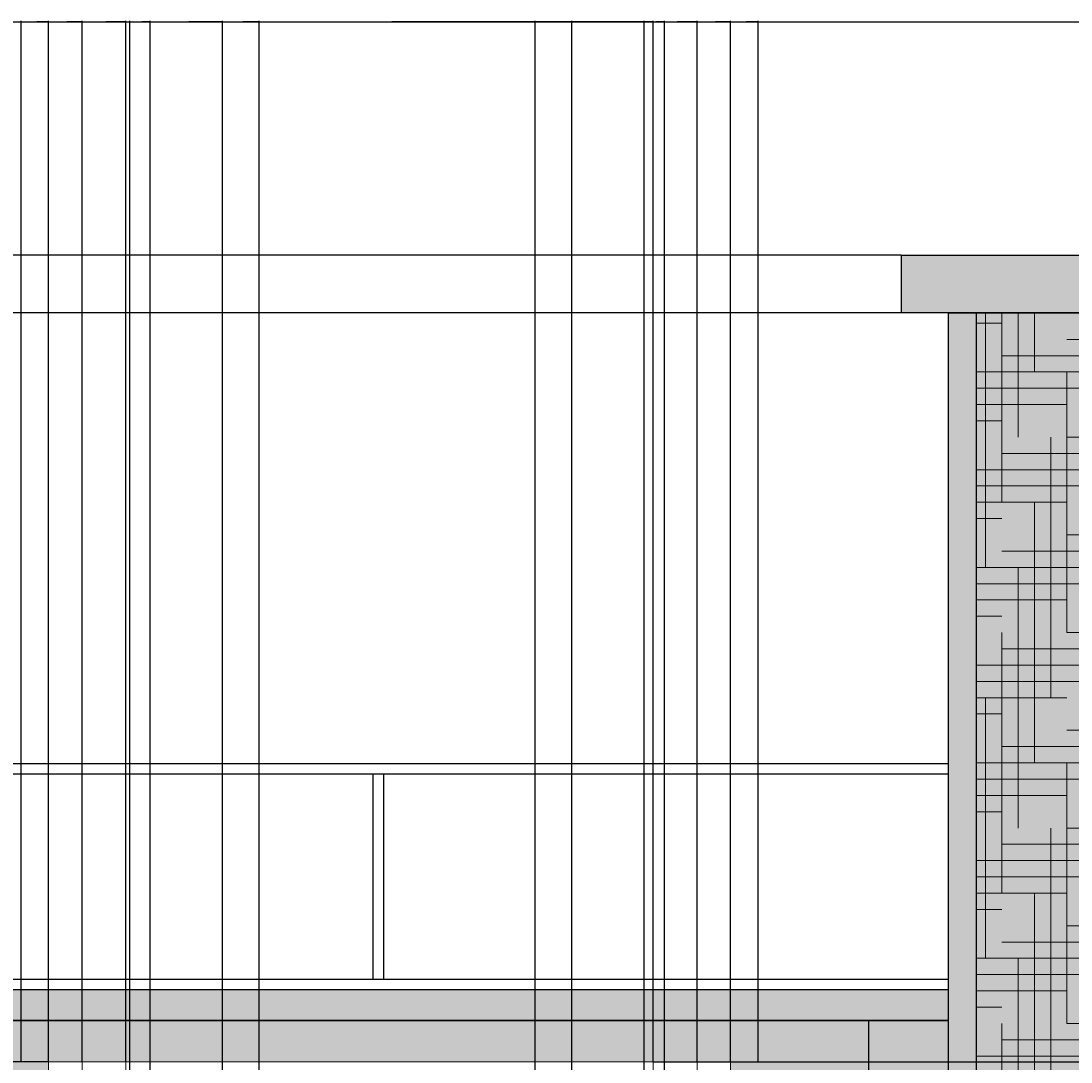
# Model space of a CAD drawing. Units: inches. Extents: x 3024 to 4744, y 1110 to 2100.
# Tile 25 of 29: x 3149 to 3354, y 1897 to 2100. Entities that reach past the tile are written whole.
import ezdxf

# ---------------------------------------------------------------- set-up
doc = ezdxf.new("R2010")
doc.units = ezdxf.units.IN
for name, color, linetype, lineweight in [('A-ANNO-DIMS', 2, 'Continuous', 18), ('A-ELEV', 7, 'Continuous', 25), ('A-ELEV-PATT', 252, 'Continuous', 13), ('A-GLAZ', 4, 'Continuous', 18)]:
    doc.layers.add(name, color=color, linetype=linetype, lineweight=lineweight)
doc.styles.get("Standard").update_dxf_attribs({"font": 'arial.ttf'})
doc.dimstyles.get("Standard").update_dxf_attribs({"dimtxt": 0.18, "dimasz": 0.18, "dimexe": 0.18, "dimexo": 0.0625, "dimgap": 0.09, "dimtad": 0, "dimtih": 1, "dimtoh": 1, "dimdec": 1, "dimzin": 0, "dimdsep": 46, "dimlunit": 3, "dimtxsty": 'Standard', "dimcen": 0.09, "dimadec": 0, "dimazin": 0, "dimtfac": 1, "dimtdec": 1, "dimtofl": 0, "dimtmove": 0, "dimatfit": 3, "dimfxl": 1, "dimtolj": 1, "dimtzin": 0, "dimarcsym": 0})

# ---------------------------------------------------------------- blocks, each defined once
blk = doc.blocks.new('WIN-BALCONY-A')
for p, q in [((3169.4, 1897.49), (3148.97, 1897.49)), ((3169.4, 1897.49), (3148.97, 1897.49)), ((3169.4, 1897.49), (3292.61, 1897.49)), ((3169.4, 1897.49), (3292.61, 1897.49)), ((3169.4, 1795.04), (3148.97, 1795.04)), ((3169.4, 1795.04), (3148.97, 1795.04)), ((3169.4, 1795.04), (3292.61, 1795.04)), ((3169.4, 1795.04), (3292.61, 1795.04))]:
    blk.add_line(p, q)
for points in [[(3148.97, 1897.49), (3148.97, 1905.61), (3292.61, 1905.61), (3292.61, 1897.49)], [(3148.97, 1897.49), (3148.97, 1905.61), (3292.61, 1905.61), (3292.61, 1897.49)], [(3292.61, 1795.04), (3292.61, 1785.61), (3148.97, 1785.61), (3148.97, 1795.04)], [(3292.61, 1795.04), (3292.61, 1785.61), (3148.97, 1785.61), (3148.97, 1795.04)]]:
    blk.add_lwpolyline(points)
for points in [[(3154.33, 1806.87), (3160.86, 1806.87), (3160.86, 1897.49), (3154.33, 1897.49)], [(3154.33, 1806.87), (3160.86, 1806.87), (3160.86, 1897.49), (3154.33, 1897.49)], [(3272.18, 1795.04), (3169.4, 1795.04), (3169.4, 1897.49), (3272.18, 1897.49)], [(3272.18, 1795.04), (3169.4, 1795.04), (3169.4, 1897.49), (3272.18, 1897.49)], [(3287.25, 1806.87), (3280.72, 1806.87), (3280.72, 1897.49), (3287.25, 1897.49)], [(3287.25, 1806.87), (3280.72, 1806.87), (3280.72, 1897.49), (3287.25, 1897.49)], [(3268.18, 1799.04), (3173.4, 1799.04), (3173.4, 1893.49), (3268.18, 1893.49)], [(3268.18, 1799.04), (3173.4, 1799.04), (3173.4, 1893.49), (3268.18, 1893.49)], [(3220.05, 1893.49), (3221.52, 1893.49), (3221.52, 1799.04), (3220.05, 1799.04)], [(3220.05, 1893.49), (3221.52, 1893.49), (3221.52, 1799.04), (3220.05, 1799.04)], [(3163.53, 1795.04), (3151.66, 1795.04), (3151.66, 1806.87), (3163.53, 1806.87)], [(3163.53, 1795.04), (3151.66, 1795.04), (3151.66, 1806.87), (3163.53, 1806.87)], [(3276.51, 1795.04), (3288.38, 1795.04), (3288.38, 1806.87), (3276.51, 1806.87)], [(3276.51, 1795.04), (3288.38, 1795.04), (3288.38, 1806.87), (3276.51, 1806.87)]]:
    blk.add_lwpolyline(points, close=True)
blk = doc.blocks.new('*D7')
at = {"layer": 'A-ANNO-DIMS', "color": 0, "lineweight": -2, "transparency": 16777216}
for p, q in [((3292.67, 1905.61), (3314.33, 1905.61)), ((3314.15, 1905.43), (3314.15, 1845.79)), ((3314.15, 1785.79), (3314.15, 1845.43)), ((3292.67, 1785.61), (3314.33, 1785.61))]:
    blk.add_line(p, q, dxfattribs=at)
at = {"layer": 'A-ANNO-DIMS', "color": 0, "transparency": 16777216}
for points in [[(3314.12, 1905.43), (3314.18, 1905.43), (3314.15, 1905.61)], [(3314.12, 1785.79), (3314.18, 1785.79), (3314.15, 1785.61)]]:
    blk.add_solid(points, dxfattribs=at)
at = {"layer": 'Defpoints', "color": 0, "transparency": 16777216}
for p in [(3292.61, 1905.61), (3314.15, 1905.61), (3292.61, 1785.61)]:
    blk.add_point(p, dxfattribs=at)
at = {"layer": 'A-ANNO-DIMS', "color": 0, "transparency": 16777216, "insert": (3314.15, 1845.61), "char_height": 0.18, "attachment_point": 5}
blk.add_mtext('\\A1;120 TYP.', dxfattribs=at)
blk = doc.blocks.new('*D64')
at = {"layer": 'A-ANNO-DIMS', "color": 0, "lineweight": -2, "transparency": 16777216}
for p, q in [((3069.79, 1241.5), (3069.79, 2100.44)), ((3069.97, 2100.26), (3405.08, 2100.26)), ((3740.97, 2100.26), (3405.87, 2100.26)), ((3741.15, 1241.5), (3741.15, 2100.44))]:
    blk.add_line(p, q, dxfattribs=at)
at = {"layer": 'A-ANNO-DIMS', "color": 0, "transparency": 16777216}
for points in [[(3069.97, 2100.29), (3069.97, 2100.23), (3069.79, 2100.26)], [(3740.97, 2100.29), (3740.97, 2100.23), (3741.15, 2100.26)]]:
    blk.add_solid(points, dxfattribs=at)
at = {"layer": 'Defpoints', "color": 0, "transparency": 16777216}
for p in [(3741.15, 2100.26), (3069.79, 1241.43), (3741.15, 1241.43)]:
    blk.add_point(p, dxfattribs=at)
at = {"layer": 'A-ANNO-DIMS', "color": 0, "transparency": 16777216, "insert": (3405.47, 2100.26), "char_height": 0.18, "attachment_point": 5}
blk.add_mtext('\\A1;671.4', dxfattribs=at)
blk = doc.blocks.new('*D73')
at = {"layer": 'A-ANNO-DIMS', "color": 0, "lineweight": -2, "transparency": 16777216}
for p, q in [((3329.64, 2043.53), (3024.11, 2043.53)), ((3024.29, 2043.35), (3024.29, 1999.76)), ((3024.29, 1955.8), (3024.29, 1999.39)), ((3105.41, 1955.62), (3024.11, 1955.62))]:
    blk.add_line(p, q, dxfattribs=at)
at = {"layer": 'A-ANNO-DIMS', "color": 0, "transparency": 16777216}
for points in [[(3024.26, 2043.35), (3024.32, 2043.35), (3024.29, 2043.53)], [(3024.26, 1955.8), (3024.32, 1955.8), (3024.29, 1955.62)]]:
    blk.add_solid(points, dxfattribs=at)
at = {"layer": 'Defpoints', "color": 0, "transparency": 16777216}
for p in [(3024.29, 2043.53), (3329.7, 2043.53), (3105.47, 1955.62)]:
    blk.add_point(p, dxfattribs=at)
at = {"layer": 'A-ANNO-DIMS', "color": 0, "transparency": 16777216, "insert": (3024.29, 1999.57), "char_height": 0.18, "attachment_point": 5}
blk.add_mtext('\\A1;87.91', dxfattribs=at)
blk = doc.blocks.new('*D74')
at = {"layer": 'A-ANNO-DIMS', "color": 0, "lineweight": -2, "transparency": 16777216}
for p, q in [((3320.5, 2054.76), (3024.11, 2054.76)), ((3024.29, 2054.58), (3024.29, 2049.33)), ((3024.29, 2043.71), (3024.29, 2048.96)), ((3320.5, 2043.53), (3024.11, 2043.53))]:
    blk.add_line(p, q, dxfattribs=at)
at = {"layer": 'A-ANNO-DIMS', "color": 0, "transparency": 16777216}
for points in [[(3024.26, 2054.58), (3024.32, 2054.58), (3024.29, 2054.76)], [(3024.26, 2043.71), (3024.32, 2043.71), (3024.29, 2043.53)]]:
    blk.add_solid(points, dxfattribs=at)
at = {"layer": 'Defpoints', "color": 0, "transparency": 16777216}
for p in [(3024.29, 2054.76), (3320.57, 2054.76), (3320.57, 2043.53)]:
    blk.add_point(p, dxfattribs=at)
at = {"layer": 'A-ANNO-DIMS', "color": 0, "transparency": 16777216, "insert": (3024.29, 2049.14), "char_height": 0.18, "attachment_point": 5}
blk.add_mtext('\\A1;11.23', dxfattribs=at)
blk = doc.blocks.new('*D82')
at = {"layer": 'A-ANNO-DIMS', "color": 0, "lineweight": -2, "transparency": 16777216}
for p, q in [((3148.97, 1897.55), (3148.97, 2100.44)), ((3149.15, 2100.26), (3151.26, 2100.26)), ((3154.15, 2100.26), (3152.04, 2100.26)), ((3154.33, 1897.55), (3154.33, 2100.44))]:
    blk.add_line(p, q, dxfattribs=at)
at = {"layer": 'A-ANNO-DIMS', "color": 0, "transparency": 16777216}
for points in [[(3149.15, 2100.29), (3149.15, 2100.23), (3148.97, 2100.26)], [(3154.15, 2100.29), (3154.15, 2100.23), (3154.33, 2100.26)]]:
    blk.add_solid(points, dxfattribs=at)
at = {"layer": 'Defpoints', "color": 0, "transparency": 16777216}
for p in [(3154.33, 2100.26), (3148.97, 1897.49), (3154.33, 1897.49)]:
    blk.add_point(p, dxfattribs=at)
at = {"layer": 'A-ANNO-DIMS', "color": 0, "transparency": 16777216, "insert": (3151.65, 2100.26), "char_height": 0.18, "attachment_point": 5}
blk.add_mtext('\\A1;5.359', dxfattribs=at)
blk = doc.blocks.new('*D83')
at = {"layer": 'A-ANNO-DIMS', "color": 0, "lineweight": -2, "transparency": 16777216}
for p, q in [((3154.33, 1897.55), (3154.33, 2100.44)), ((3154.51, 2100.26), (3157.27, 2100.26)), ((3160.68, 2100.26), (3157.92, 2100.26)), ((3160.86, 1897.55), (3160.86, 2100.44))]:
    blk.add_line(p, q, dxfattribs=at)
at = {"layer": 'A-ANNO-DIMS', "color": 0, "transparency": 16777216}
for points in [[(3154.51, 2100.29), (3154.51, 2100.23), (3154.33, 2100.26)], [(3160.68, 2100.29), (3160.68, 2100.23), (3160.86, 2100.26)]]:
    blk.add_solid(points, dxfattribs=at)
at = {"layer": 'Defpoints', "color": 0, "transparency": 16777216}
for p in [(3160.86, 2100.26), (3154.33, 1897.49), (3160.86, 1897.49)]:
    blk.add_point(p, dxfattribs=at)
at = {"layer": 'A-ANNO-DIMS', "color": 0, "transparency": 16777216, "insert": (3157.59, 2100.26), "char_height": 0.18, "attachment_point": 5}
blk.add_mtext('\\A1;6.53', dxfattribs=at)
blk = doc.blocks.new('*D84')
at = {"layer": 'A-ANNO-DIMS', "color": 0, "lineweight": -2, "transparency": 16777216}
for p, q in [((3160.86, 1897.55), (3160.86, 2100.44)), ((3161.04, 2100.26), (3164.73, 2100.26)), ((3169.22, 2100.26), (3165.52, 2100.26)), ((3169.4, 1897.55), (3169.4, 2100.44))]:
    blk.add_line(p, q, dxfattribs=at)
at = {"layer": 'A-ANNO-DIMS', "color": 0, "transparency": 16777216}
for points in [[(3161.04, 2100.29), (3161.04, 2100.23), (3160.86, 2100.26)], [(3169.22, 2100.29), (3169.22, 2100.23), (3169.4, 2100.26)]]:
    blk.add_solid(points, dxfattribs=at)
at = {"layer": 'Defpoints', "color": 0, "transparency": 16777216}
for p in [(3169.4, 2100.26), (3160.86, 1897.49), (3169.4, 1897.49)]:
    blk.add_point(p, dxfattribs=at)
at = {"layer": 'A-ANNO-DIMS', "color": 0, "transparency": 16777216, "insert": (3165.13, 2100.26), "char_height": 0.18, "attachment_point": 5}
blk.add_mtext('\\A1;8.538', dxfattribs=at)
blk = doc.blocks.new('*D85')
at = {"layer": 'A-ANNO-DIMS', "color": 0, "lineweight": -2, "transparency": 16777216}
for p, q in [((3169.4, 1897.55), (3169.4, 2100.44)), ((3169.58, 2100.26), (3220.33, 2100.26)), ((3272, 2100.26), (3221.24, 2100.26)), ((3272.18, 1897.55), (3272.18, 2100.44))]:
    blk.add_line(p, q, dxfattribs=at)
at = {"layer": 'A-ANNO-DIMS', "color": 0, "transparency": 16777216}
for points in [[(3169.58, 2100.29), (3169.58, 2100.23), (3169.4, 2100.26)], [(3272, 2100.29), (3272, 2100.23), (3272.18, 2100.26)]]:
    blk.add_solid(points, dxfattribs=at)
at = {"layer": 'Defpoints', "color": 0, "transparency": 16777216}
for p in [(3272.18, 2100.26), (3169.4, 1897.49), (3272.18, 1897.49)]:
    blk.add_point(p, dxfattribs=at)
at = {"layer": 'A-ANNO-DIMS', "color": 0, "transparency": 16777216, "insert": (3220.79, 2100.26), "char_height": 0.18, "attachment_point": 5}
blk.add_mtext('\\A1;102.78', dxfattribs=at)
blk = doc.blocks.new('*D86')
at = {"layer": 'A-ANNO-DIMS', "color": 0, "lineweight": -2, "transparency": 16777216}
for p, q in [((3272.18, 1897.55), (3272.18, 2100.44)), ((3272.36, 2100.26), (3276.05, 2100.26)), ((3280.54, 2100.26), (3276.84, 2100.26)), ((3280.72, 1897.55), (3280.72, 2100.44))]:
    blk.add_line(p, q, dxfattribs=at)
at = {"layer": 'A-ANNO-DIMS', "color": 0, "transparency": 16777216}
for points in [[(3272.36, 2100.29), (3272.36, 2100.23), (3272.18, 2100.26)], [(3280.54, 2100.29), (3280.54, 2100.23), (3280.72, 2100.26)]]:
    blk.add_solid(points, dxfattribs=at)
at = {"layer": 'Defpoints', "color": 0, "transparency": 16777216}
for p in [(3280.72, 2100.26), (3272.18, 1897.49), (3280.72, 1897.49)]:
    blk.add_point(p, dxfattribs=at)
at = {"layer": 'A-ANNO-DIMS', "color": 0, "transparency": 16777216, "insert": (3276.45, 2100.26), "char_height": 0.18, "attachment_point": 5}
blk.add_mtext('\\A1;8.538', dxfattribs=at)
blk = doc.blocks.new('*D87')
at = {"layer": 'A-ANNO-DIMS', "color": 0, "lineweight": -2, "transparency": 16777216}
for p, q in [((3280.72, 1897.55), (3280.72, 2100.44)), ((3280.9, 2100.26), (3283.66, 2100.26)), ((3287.07, 2100.26), (3284.31, 2100.26)), ((3287.25, 1897.55), (3287.25, 2100.44))]:
    blk.add_line(p, q, dxfattribs=at)
at = {"layer": 'A-ANNO-DIMS', "color": 0, "transparency": 16777216}
for points in [[(3280.9, 2100.29), (3280.9, 2100.23), (3280.72, 2100.26)], [(3287.07, 2100.29), (3287.07, 2100.23), (3287.25, 2100.26)]]:
    blk.add_solid(points, dxfattribs=at)
at = {"layer": 'Defpoints', "color": 0, "transparency": 16777216}
for p in [(3287.25, 2100.26), (3280.72, 1897.49), (3287.25, 1897.49)]:
    blk.add_point(p, dxfattribs=at)
at = {"layer": 'A-ANNO-DIMS', "color": 0, "transparency": 16777216, "insert": (3283.98, 2100.26), "char_height": 0.18, "attachment_point": 5}
blk.add_mtext('\\A1;6.53', dxfattribs=at)
blk = doc.blocks.new('*D88')
at = {"layer": 'A-ANNO-DIMS', "color": 0, "lineweight": -2, "transparency": 16777216}
for p, q in [((3287.25, 1897.55), (3287.25, 2100.44)), ((3287.43, 2100.26), (3289.53, 2100.26)), ((3292.43, 2100.26), (3290.32, 2100.26)), ((3292.61, 1897.55), (3292.61, 2100.44))]:
    blk.add_line(p, q, dxfattribs=at)
at = {"layer": 'A-ANNO-DIMS', "color": 0, "transparency": 16777216}
for points in [[(3287.43, 2100.29), (3287.43, 2100.23), (3287.25, 2100.26)], [(3292.43, 2100.29), (3292.43, 2100.23), (3292.61, 2100.26)]]:
    blk.add_solid(points, dxfattribs=at)
at = {"layer": 'Defpoints', "color": 0, "transparency": 16777216}
for p in [(3292.61, 2100.26), (3287.25, 1897.49), (3292.61, 1897.49)]:
    blk.add_point(p, dxfattribs=at)
at = {"layer": 'A-ANNO-DIMS', "color": 0, "transparency": 16777216, "insert": (3289.93, 2100.26), "char_height": 0.18, "attachment_point": 5}
blk.add_mtext('\\A1;5.359', dxfattribs=at)
blk = doc.blocks.new('*D98')
at = {"layer": 'A-ANNO-DIMS', "color": 0, "lineweight": -2, "transparency": 16777216}
for p, q in [((3154.27, 1897.49), (3024.11, 1897.49)), ((3024.29, 1897.31), (3024.29, 1852.36)), ((3024.29, 1807.05), (3024.29, 1852)), ((3154.27, 1806.87), (3024.11, 1806.87))]:
    blk.add_line(p, q, dxfattribs=at)
at = {"layer": 'A-ANNO-DIMS', "color": 0, "transparency": 16777216}
for points in [[(3024.26, 1897.31), (3024.32, 1897.31), (3024.29, 1897.49)], [(3024.26, 1807.05), (3024.32, 1807.05), (3024.29, 1806.87)]]:
    blk.add_solid(points, dxfattribs=at)
at = {"layer": 'Defpoints', "color": 0, "transparency": 16777216}
for p in [(3024.29, 1897.49), (3154.33, 1897.49), (3154.33, 1806.87)]:
    blk.add_point(p, dxfattribs=at)
at = {"layer": 'A-ANNO-DIMS', "color": 0, "transparency": 16777216, "insert": (3024.29, 1852.18), "char_height": 0.18, "attachment_point": 5}
blk.add_mtext('\\A1;90.62', dxfattribs=at)
blk = doc.blocks.new('*D102')
at = {"layer": 'A-ANNO-DIMS', "color": 0, "lineweight": -2, "transparency": 16777216}
for p, q in [((3272.24, 1897.49), (3786.83, 1897.49)), ((3786.65, 1897.31), (3786.65, 1895.67)), ((3786.65, 1893.67), (3786.65, 1895.31)), ((3268.24, 1893.49), (3786.83, 1893.49))]:
    blk.add_line(p, q, dxfattribs=at)
at = {"layer": 'A-ANNO-DIMS', "color": 0, "transparency": 16777216}
for points in [[(3786.62, 1897.31), (3786.68, 1897.31), (3786.65, 1897.49)], [(3786.62, 1893.67), (3786.68, 1893.67), (3786.65, 1893.49)]]:
    blk.add_solid(points, dxfattribs=at)
at = {"layer": 'Defpoints', "color": 0, "transparency": 16777216}
for p in [(3272.18, 1897.49), (3786.65, 1897.49), (3268.18, 1893.49)]:
    blk.add_point(p, dxfattribs=at)
at = {"layer": 'A-ANNO-DIMS', "color": 0, "transparency": 16777216, "insert": (3786.65, 1895.49), "char_height": 0.18, "attachment_point": 5}
blk.add_mtext('\\A1;4.00', dxfattribs=at)
blk = doc.blocks.new('*D106')
at = {"layer": 'A-ANNO-DIMS', "color": 0, "lineweight": -2, "transparency": 16777216}
for p, q in [((3170.16, 1275.67), (3170.16, 2100.44)), ((3170.34, 2100.26), (3171.83, 2100.26)), ((3173.98, 2100.26), (3172.49, 2100.26)), ((3174.16, 1271.67), (3174.16, 2100.44))]:
    blk.add_line(p, q, dxfattribs=at)
at = {"layer": 'A-ANNO-DIMS', "color": 0, "transparency": 16777216}
for points in [[(3170.34, 2100.29), (3170.34, 2100.23), (3170.16, 2100.26)], [(3173.98, 2100.29), (3173.98, 2100.23), (3174.16, 2100.26)]]:
    blk.add_solid(points, dxfattribs=at)
at = {"layer": 'Defpoints', "color": 0, "transparency": 16777216}
for p in [(3174.16, 2100.26), (3170.16, 1275.61), (3174.16, 1271.61)]:
    blk.add_point(p, dxfattribs=at)
at = {"layer": 'A-ANNO-DIMS', "color": 0, "transparency": 16777216, "insert": (3172.16, 2100.26), "char_height": 0.18, "attachment_point": 5}
blk.add_mtext('\\A1;4.00', dxfattribs=at)
blk = doc.blocks.new('*D107')
at = {"layer": 'A-ANNO-DIMS', "color": 0, "lineweight": -2, "transparency": 16777216}
for p, q in [((3174.16, 1271.67), (3174.16, 2100.44)), ((3174.34, 2100.26), (3221.88, 2100.26)), ((3270.21, 2100.26), (3222.67, 2100.26)), ((3270.39, 1271.67), (3270.39, 2100.44))]:
    blk.add_line(p, q, dxfattribs=at)
at = {"layer": 'A-ANNO-DIMS', "color": 0, "transparency": 16777216}
for points in [[(3174.34, 2100.29), (3174.34, 2100.23), (3174.16, 2100.26)], [(3270.21, 2100.29), (3270.21, 2100.23), (3270.39, 2100.26)]]:
    blk.add_solid(points, dxfattribs=at)
at = {"layer": 'Defpoints', "color": 0, "transparency": 16777216}
for p in [(3270.39, 2100.26), (3174.16, 1271.61), (3270.39, 1271.61)]:
    blk.add_point(p, dxfattribs=at)
at = {"layer": 'A-ANNO-DIMS', "color": 0, "transparency": 16777216, "insert": (3222.27, 2100.26), "char_height": 0.18, "attachment_point": 5}
blk.add_mtext('\\A1;96.23', dxfattribs=at)
blk = doc.blocks.new('*D108')
at = {"layer": 'A-ANNO-DIMS', "color": 0, "lineweight": -2, "transparency": 16777216}
for p, q in [((3270.39, 1271.67), (3270.39, 2100.44)), ((3270.57, 2100.26), (3272.06, 2100.26)), ((3274.21, 2100.26), (3272.71, 2100.26)), ((3274.39, 1275.67), (3274.39, 2100.44))]:
    blk.add_line(p, q, dxfattribs=at)
at = {"layer": 'A-ANNO-DIMS', "color": 0, "transparency": 16777216}
for points in [[(3270.57, 2100.29), (3270.57, 2100.23), (3270.39, 2100.26)], [(3274.21, 2100.29), (3274.21, 2100.23), (3274.39, 2100.26)]]:
    blk.add_solid(points, dxfattribs=at)
at = {"layer": 'Defpoints', "color": 0, "transparency": 16777216}
for p in [(3274.39, 2100.26), (3274.39, 1275.61), (3270.39, 1271.61)]:
    blk.add_point(p, dxfattribs=at)
at = {"layer": 'A-ANNO-DIMS', "color": 0, "transparency": 16777216, "insert": (3272.39, 2100.26), "char_height": 0.18, "attachment_point": 5}
blk.add_mtext('\\A1;4.00', dxfattribs=at)
blk = doc.blocks.new('*D124')
at = {"layer": 'A-ANNO-DIMS', "color": 0, "lineweight": -2, "transparency": 16777216}
for p, q in [((3174.16, 1271.67), (3174.16, 2100.44)), ((3174.34, 2100.26), (3180.75, 2100.26)), ((3188.08, 2100.26), (3181.67, 2100.26)), ((3188.26, 1256.29), (3188.26, 2100.44))]:
    blk.add_line(p, q, dxfattribs=at)
at = {"layer": 'A-ANNO-DIMS', "color": 0, "transparency": 16777216}
for points in [[(3174.34, 2100.29), (3174.34, 2100.23), (3174.16, 2100.26)], [(3188.08, 2100.29), (3188.08, 2100.23), (3188.26, 2100.26)]]:
    blk.add_solid(points, dxfattribs=at)
at = {"layer": 'Defpoints', "color": 0, "transparency": 16777216}
for p in [(3188.26, 2100.26), (3174.16, 1271.61), (3188.26, 1256.23)]:
    blk.add_point(p, dxfattribs=at)
at = {"layer": 'A-ANNO-DIMS', "color": 0, "transparency": 16777216, "insert": (3181.21, 2100.26), "char_height": 0.18, "attachment_point": 5}
blk.add_mtext('\\A1;14.098', dxfattribs=at)
blk = doc.blocks.new('*D125')
at = {"layer": 'A-ANNO-DIMS', "color": 0, "lineweight": -2, "transparency": 16777216}
for p, q in [((3188.26, 1256.29), (3188.26, 2100.44)), ((3188.44, 2100.26), (3191.44, 2100.26)), ((3195.23, 2100.26), (3192.22, 2100.26)), ((3195.41, 1256.29), (3195.41, 2100.44))]:
    blk.add_line(p, q, dxfattribs=at)
at = {"layer": 'A-ANNO-DIMS', "color": 0, "transparency": 16777216}
for points in [[(3188.44, 2100.29), (3188.44, 2100.23), (3188.26, 2100.26)], [(3195.23, 2100.29), (3195.23, 2100.23), (3195.41, 2100.26)]]:
    blk.add_solid(points, dxfattribs=at)
at = {"layer": 'Defpoints', "color": 0, "transparency": 16777216}
for p in [(3195.41, 2100.26), (3188.26, 1256.23), (3195.41, 1256.23)]:
    blk.add_point(p, dxfattribs=at)
at = {"layer": 'A-ANNO-DIMS', "color": 0, "transparency": 16777216, "insert": (3191.83, 2100.26), "char_height": 0.18, "attachment_point": 5}
blk.add_mtext('\\A1;7.147', dxfattribs=at)
blk = doc.blocks.new('*D126')
at = {"layer": 'A-ANNO-DIMS', "color": 0, "lineweight": -2, "transparency": 16777216}
for p, q in [((3249.14, 1256.29), (3249.14, 2100.44)), ((3249.32, 2100.26), (3252.32, 2100.26)), ((3256.11, 2100.26), (3253.11, 2100.26)), ((3256.29, 1256.29), (3256.29, 2100.44))]:
    blk.add_line(p, q, dxfattribs=at)
at = {"layer": 'A-ANNO-DIMS', "color": 0, "transparency": 16777216}
for points in [[(3249.32, 2100.29), (3249.32, 2100.23), (3249.14, 2100.26)], [(3256.11, 2100.29), (3256.11, 2100.23), (3256.29, 2100.26)]]:
    blk.add_solid(points, dxfattribs=at)
at = {"layer": 'Defpoints', "color": 0, "transparency": 16777216}
for p in [(3256.29, 2100.26), (3249.14, 1256.23), (3256.29, 1256.23)]:
    blk.add_point(p, dxfattribs=at)
at = {"layer": 'A-ANNO-DIMS', "color": 0, "transparency": 16777216, "insert": (3252.72, 2100.26), "char_height": 0.18, "attachment_point": 5}
blk.add_mtext('\\A1;7.147', dxfattribs=at)

msp = doc.modelspace()

# ---------------------------------------------------------------- hatches: boundary and pattern name
at = {"layer": 'A-ELEV-PATT'}
h = msp.add_hatch(color=256, dxfattribs=at)
h.dxf.hatch_style = 1
h.paths.add_polyline_path([(3491.8271, 2054.7584), (3320.5658, 2054.7584), (3320.5658, 2043.5286), (3491.8271, 2043.5286)])
h.paths.add_polyline_path([(3292.6051, 1905.6112), (3148.9694, 1905.6112), (3148.9694, 1897.4879), (3169.3964, 1897.4879), (3292.6051, 1897.4879)])
h.paths.add_polyline_path([(3292.6051, 1795.0431), (3169.3964, 1795.0431), (3148.9694, 1795.0431), (3148.9694, 1785.6112), (3292.6051, 1785.6112)])
h.paths.add_polyline_path([(3292.6051, 1779.6112), (3148.9694, 1779.6112), (3148.9694, 1771.4879), (3169.3964, 1771.4879), (3292.6051, 1771.4879)])
h.paths.add_polyline_path([(3292.6051, 1669.0431), (3169.3964, 1669.0431), (3148.9694, 1669.0431), (3148.9694, 1659.6112), (3292.6051, 1659.6112)])
h.paths.add_polyline_path([(3292.6051, 1653.6112), (3148.9694, 1653.6112), (3148.9694, 1645.4879), (3169.3964, 1645.4879), (3292.6051, 1645.4879)])
h.paths.add_polyline_path([(3292.6051, 1543.0431), (3169.3964, 1543.0431), (3148.9694, 1543.0431), (3148.9694, 1533.6112), (3292.6051, 1533.6112)])
h.paths.add_polyline_path([(3292.6051, 1527.6112), (3148.9694, 1527.6112), (3148.9694, 1519.4879), (3169.3964, 1519.4879), (3292.6051, 1519.4879)])
h.paths.add_polyline_path([(3292.6051, 1401.6112), (3148.9694, 1401.6112), (3148.9694, 1393.4879), (3169.3964, 1393.4879), (3292.6051, 1393.4879)])
h.paths.add_polyline_path([(3292.6051, 1417.0431), (3169.3964, 1417.0431), (3148.9694, 1417.0431), (3148.9694, 1407.6112), (3292.6051, 1407.6112)])
h.paths.add_polyline_path([(3292.6051, 1291.0431), (3169.3964, 1291.0431), (3148.9694, 1291.0431), (3148.9694, 1281.6112), (3292.6051, 1281.6112)])
h.paths.add_polyline_path([(3654.037, 1165.0431), (3530.8283, 1165.0431), (3510.4013, 1165.0431), (3510.4013, 1155.6112), (3654.037, 1155.6112)])
h.paths.add_polyline_path([(3654.037, 1275.6112), (3510.4013, 1275.6112), (3510.4013, 1267.4879), (3530.8283, 1267.4879), (3654.037, 1267.4879)])
h.paths.add_polyline_path([(3654.037, 1291.0431), (3530.8283, 1291.0431), (3510.4013, 1291.0431), (3510.4013, 1281.6112), (3654.037, 1281.6112)])
h.paths.add_polyline_path([(3654.037, 1417.0431), (3530.8283, 1417.0431), (3510.4013, 1417.0431), (3510.4013, 1407.6112), (3654.037, 1407.6112)])
h.paths.add_polyline_path([(3654.037, 1401.6112), (3510.4013, 1401.6112), (3510.4013, 1393.4879), (3530.8283, 1393.4879), (3654.037, 1393.4879)])
h.paths.add_polyline_path([(3654.037, 1543.0431), (3530.8283, 1543.0431), (3510.4013, 1543.0431), (3510.4013, 1533.6112), (3654.037, 1533.6112)])
h.paths.add_polyline_path([(3654.037, 1527.6112), (3510.4013, 1527.6112), (3510.4013, 1519.4879), (3530.8283, 1519.4879), (3654.037, 1519.4879)])
h.paths.add_polyline_path([(3654.037, 1653.6112), (3510.4013, 1653.6112), (3510.4013, 1645.4879), (3530.8283, 1645.4879), (3654.037, 1645.4879)])
h.paths.add_polyline_path([(3654.037, 1669.0431), (3530.8283, 1669.0431), (3510.4013, 1669.0431), (3510.4013, 1659.6112), (3654.037, 1659.6112)])
h.paths.add_polyline_path([(3654.037, 1779.6112), (3510.4013, 1779.6112), (3510.4013, 1771.4879), (3530.8283, 1771.4879), (3654.037, 1771.4879)])
h.paths.add_polyline_path([(3654.037, 1795.0431), (3530.8283, 1795.0431), (3510.4013, 1795.0431), (3510.4013, 1785.6112), (3654.037, 1785.6112)])
h.paths.add_polyline_path([(3654.037, 1905.6112), (3510.4013, 1905.6112), (3510.4013, 1897.4879), (3530.8283, 1897.4879), (3654.037, 1897.4879)])
h = msp.add_hatch(color=256, dxfattribs=at)
h.dxf.hatch_style = 1
h.paths.add_polyline_path([(3335.1044, 2043.5286), (3329.7033, 2043.5286), (3329.7033, 1155.6112), (3335.1044, 1155.6112)])
h.paths.add_polyline_path([(3481.2411, 2043.5286), (3335.1044, 2043.5286), (3335.1044, 1155.6112), (3481.2411, 1155.6112)])
h.paths.add_polyline_path([(3449.7202, 1329.5246), (3361.2242, 1329.5246), (3361.2242, 1436.6064), (3449.7202, 1436.6064)], flags=16)
h.paths.add_polyline_path([(3445.7202, 1333.5246), (3365.2242, 1333.5246), (3365.2242, 1432.6064), (3445.7202, 1432.6064)], flags=0)
h.paths.add_polyline_path([(3449.7202, 1455.5246), (3361.2242, 1455.5246), (3361.2242, 1562.6064), (3449.7202, 1562.6064)], flags=16)
h.paths.add_polyline_path([(3445.7202, 1459.5246), (3365.2242, 1459.5246), (3365.2242, 1558.6064), (3445.7202, 1558.6064)], flags=0)
h.paths.add_polyline_path([(3449.7202, 1581.5246), (3361.2242, 1581.5246), (3361.2242, 1688.6064), (3449.7202, 1688.6064)], flags=16)
h.paths.add_polyline_path([(3445.7202, 1585.5246), (3365.2242, 1585.5246), (3365.2242, 1684.6064), (3445.7202, 1684.6064)], flags=0)
h.paths.add_polyline_path([(3449.7202, 1707.5246), (3361.2242, 1707.5246), (3361.2242, 1814.6064), (3449.7202, 1814.6064)], flags=16)
h.paths.add_polyline_path([(3445.7202, 1711.5246), (3365.2242, 1711.5246), (3365.2242, 1810.6064), (3445.7202, 1810.6064)], flags=0)
h.paths.add_polyline_path([(3449.7202, 1833.5246), (3361.2242, 1833.5246), (3361.2242, 1940.6064), (3449.7202, 1940.6064)], flags=16)
h.paths.add_polyline_path([(3445.7202, 1837.5246), (3365.2242, 1837.5246), (3365.2242, 1936.6064), (3445.7202, 1936.6064)], flags=0)
h = msp.add_hatch(color=256, dxfattribs=at)
h.dxf.hatch_style = 1
h.paths.add_polyline_path([(3475.84, 2043.5286), (3335.1044, 2043.5286), (3335.1044, 1155.6112), (3475.84, 1155.6112)])
h.paths.add_polyline_path([(3449.7202, 1940.6064), (3449.7202, 1833.5246), (3361.2242, 1833.5246), (3361.2242, 1940.6064)], flags=16)
h.paths.add_polyline_path([(3445.7202, 1936.6064), (3445.7202, 1837.5246), (3365.2242, 1837.5246), (3365.2242, 1936.6064)], flags=0)
h.paths.add_polyline_path([(3449.7202, 1814.6064), (3449.7202, 1707.5246), (3361.2242, 1707.5246), (3361.2242, 1814.6064)], flags=16)
h.paths.add_polyline_path([(3445.7202, 1810.6064), (3445.7202, 1711.5246), (3365.2242, 1711.5246), (3365.2242, 1810.6064)], flags=0)
h.paths.add_polyline_path([(3449.7202, 1688.6064), (3449.7202, 1581.5246), (3361.2242, 1581.5246), (3361.2242, 1688.6064)], flags=16)
h.paths.add_polyline_path([(3445.7202, 1684.6064), (3445.7202, 1585.5246), (3365.2242, 1585.5246), (3365.2242, 1684.6064)], flags=0)
h.paths.add_polyline_path([(3449.7202, 1562.6064), (3449.7202, 1455.5246), (3361.2242, 1455.5246), (3361.2242, 1562.6064)], flags=16)
h.paths.add_polyline_path([(3445.7202, 1558.6064), (3445.7202, 1459.5246), (3365.2242, 1459.5246), (3365.2242, 1558.6064)], flags=0)
h.paths.add_polyline_path([(3449.7202, 1436.6064), (3449.7202, 1329.5246), (3361.2242, 1329.5246), (3361.2242, 1436.6064)], flags=16)
h.paths.add_polyline_path([(3445.7202, 1432.6064), (3445.7202, 1333.5246), (3365.2242, 1333.5246), (3365.2242, 1432.6064)], flags=0)
h = msp.add_hatch(dxfattribs=at)
h.set_pattern_fill('HOUND', color=256, scale=2)
h.paths.add_polyline_path([(3475.84, 2043.5286), (3335.1044, 2043.5286), (3335.1044, 1155.6112), (3475.84, 1155.6112)])
h.paths.add_polyline_path([(3449.7202, 1940.6064), (3449.7202, 1833.5246), (3361.2242, 1833.5246), (3361.2242, 1940.6064)], flags=16)
h.paths.add_polyline_path([(3445.7202, 1936.6064), (3445.7202, 1837.5246), (3365.2242, 1837.5246), (3365.2242, 1936.6064)], flags=0)
h.paths.add_polyline_path([(3449.7202, 1814.6064), (3449.7202, 1707.5246), (3361.2242, 1707.5246), (3361.2242, 1814.6064)], flags=16)
h.paths.add_polyline_path([(3445.7202, 1810.6064), (3445.7202, 1711.5246), (3365.2242, 1711.5246), (3365.2242, 1810.6064)], flags=0)
h.paths.add_polyline_path([(3449.7202, 1688.6064), (3449.7202, 1581.5246), (3361.2242, 1581.5246), (3361.2242, 1688.6064)], flags=16)
h.paths.add_polyline_path([(3445.7202, 1684.6064), (3445.7202, 1585.5246), (3365.2242, 1585.5246), (3365.2242, 1684.6064)], flags=0)
h.paths.add_polyline_path([(3449.7202, 1562.6064), (3449.7202, 1455.5246), (3361.2242, 1455.5246), (3361.2242, 1562.6064)], flags=16)
h.paths.add_polyline_path([(3445.7202, 1558.6064), (3445.7202, 1459.5246), (3365.2242, 1459.5246), (3365.2242, 1558.6064)], flags=0)
h.paths.add_polyline_path([(3449.7202, 1436.6064), (3449.7202, 1329.5246), (3361.2242, 1329.5246), (3361.2242, 1436.6064)], flags=16)
h.paths.add_polyline_path([(3445.7202, 1432.6064), (3445.7202, 1333.5246), (3365.2242, 1333.5246), (3365.2242, 1432.6064)], flags=0)
h = msp.add_hatch(color=256, dxfattribs=at)
h.dxf.hatch_style = 1
h.paths.add_polyline_path([(3221.5241, 2019.4879), (3220.0505, 2019.4879), (3220.0505, 1925.0431), (3221.5241, 1925.0431)], flags=0)
h.paths.add_polyline_path([(3221.5241, 2019.4879), (3221.5241, 1925.0431), (3220.0505, 1925.0431), (3220.0505, 2019.4879)], flags=0)
h.paths.add_polyline_path([(3221.5241, 1893.4879), (3220.0505, 1893.4879), (3220.0505, 1799.0431), (3221.5241, 1799.0431)])
h = msp.add_hatch(color=256, dxfattribs=at)
h.dxf.hatch_style = 1
h.paths.add_polyline_path([(3329.7033, 1407.6112), (3105.4722, 1407.6112), (3105.4722, 1401.6112), (3329.7033, 1401.6112)])
h.paths.add_polyline_path([(3329.7033, 1281.6112), (3105.4722, 1281.6112), (3105.4722, 1275.6112), (3112.3838, 1275.6112), (3329.7033, 1275.6112)])
h.paths.add_polyline_path([(3329.7033, 1533.6112), (3105.4722, 1533.6112), (3105.4722, 1527.6112), (3329.7033, 1527.6112)])
h.paths.add_polyline_path([(3329.7033, 1659.6112), (3105.4722, 1659.6112), (3105.4722, 1653.6112), (3329.7033, 1653.6112)])
h.paths.add_polyline_path([(3329.7033, 1785.6112), (3105.4722, 1785.6112), (3105.4722, 1779.6112), (3329.7033, 1779.6112)])
h.paths.add_polyline_path([(3329.7033, 1911.6112), (3105.4722, 1911.6112), (3095.7158, 1911.6112), (3095.7158, 1905.6112), (3329.7033, 1905.6112)])
h.paths.add_polyline_path([(3715.2286, 1911.6112), (3705.4722, 1911.6112), (3705.4722, 1905.6112), (3715.2286, 1905.6112)])
h.paths.add_polyline_path([(3688.5588, 1911.6112), (3481.2411, 1911.6112), (3481.2411, 1905.6112), (3688.5588, 1905.6112)])
h = msp.add_hatch(color=256, dxfattribs=at)
h.dxf.hatch_style = 1
h.paths.add_polyline_path([(3154.3287, 1897.4879), (3148.9694, 1897.4879), (3148.9694, 1905.6112), (3105.4722, 1905.6112), (3105.4722, 1785.6112), (3148.9694, 1785.6112), (3148.9694, 1795.0431), (3151.6604, 1795.0431), (3151.6604, 1806.8674), (3154.3287, 1806.8674)])
h.paths.add_polyline_path([(3329.7033, 1905.6112), (3292.6051, 1905.6112), (3292.6051, 1897.4879), (3287.2458, 1897.4879), (3287.2458, 1806.8674), (3288.3759, 1806.8674), (3288.3759, 1795.0431), (3292.6051, 1795.0431), (3292.6051, 1785.6112), (3329.7033, 1785.6112)])
h.paths.add_polyline_path([(3154.3287, 1771.4879), (3148.9694, 1771.4879), (3148.9694, 1779.6112), (3105.4722, 1779.6112), (3105.4722, 1659.6112), (3148.9694, 1659.6112), (3148.9694, 1669.0431), (3151.6604, 1669.0431), (3151.6604, 1680.8674), (3154.3287, 1680.8674)])
h.paths.add_polyline_path([(3329.7033, 1779.6112), (3292.6051, 1779.6112), (3292.6051, 1771.4879), (3287.2458, 1771.4879), (3287.2458, 1680.8674), (3288.3759, 1680.8674), (3288.3759, 1669.0431), (3292.6051, 1669.0431), (3292.6051, 1659.6112), (3329.7033, 1659.6112)])
h.paths.add_polyline_path([(3154.3287, 1645.4879), (3148.9694, 1645.4879), (3148.9694, 1653.6112), (3105.4722, 1653.6112), (3105.4722, 1533.6112), (3148.9694, 1533.6112), (3148.9694, 1543.0431), (3151.6604, 1543.0431), (3151.6604, 1554.8674), (3154.3287, 1554.8674)])
h.paths.add_polyline_path([(3329.7033, 1653.6112), (3292.6051, 1653.6112), (3292.6051, 1645.4879), (3287.2458, 1645.4879), (3287.2458, 1554.8674), (3288.3759, 1554.8674), (3288.3759, 1543.0431), (3292.6051, 1543.0431), (3292.6051, 1533.6112), (3329.7033, 1533.6112)])
h.paths.add_polyline_path([(3329.7033, 1527.6112), (3292.6051, 1527.6112), (3292.6051, 1519.4879), (3287.2458, 1519.4879), (3287.2458, 1428.8674), (3288.3759, 1428.8674), (3288.3759, 1417.0431), (3292.6051, 1417.0431), (3292.6051, 1407.6112), (3329.7033, 1407.6112)])
h.paths.add_polyline_path([(3329.7033, 1401.6112), (3292.6051, 1401.6112), (3292.6051, 1393.4879), (3287.2458, 1393.4879), (3287.2458, 1302.8674), (3288.3759, 1302.8674), (3288.3759, 1291.0431), (3292.6051, 1291.0431), (3292.6051, 1281.6112), (3329.7033, 1281.6112)])
h.paths.add_polyline_path([(3154.3287, 1393.4879), (3148.9694, 1393.4879), (3148.9694, 1401.6112), (3105.4722, 1401.6112), (3105.4722, 1281.6112), (3148.9694, 1281.6112), (3148.9694, 1291.0431), (3151.6604, 1291.0431), (3151.6604, 1302.8674), (3154.3287, 1302.8674)])
h.paths.add_polyline_path([(3154.3287, 1519.4879), (3148.9694, 1519.4879), (3148.9694, 1527.6112), (3105.4722, 1527.6112), (3105.4722, 1407.6112), (3148.9694, 1407.6112), (3148.9694, 1417.0431), (3151.6604, 1417.0431), (3151.6604, 1428.8674), (3154.3287, 1428.8674)])
h.paths.add_polyline_path([(3515.7606, 1897.4879), (3510.4013, 1897.4879), (3510.4013, 1905.6112), (3481.2411, 1905.6112), (3481.2411, 1785.6112), (3510.4013, 1785.6112), (3510.4013, 1795.0431), (3513.0923, 1795.0431), (3513.0923, 1806.8674), (3515.7606, 1806.8674)])
h.paths.add_polyline_path([(3688.5588, 1905.6112), (3654.037, 1905.6112), (3654.037, 1897.4879), (3648.6777, 1897.4879), (3648.6777, 1806.8674), (3649.8078, 1806.8674), (3649.8078, 1795.0431), (3654.037, 1795.0431), (3654.037, 1785.6112), (3688.5588, 1785.6112)])
h.paths.add_polyline_path([(3515.7606, 1771.4879), (3510.4013, 1771.4879), (3510.4013, 1779.6112), (3481.2411, 1779.6112), (3481.2411, 1659.6112), (3510.4013, 1659.6112), (3510.4013, 1669.0431), (3513.0923, 1669.0431), (3513.0923, 1680.8674), (3515.7606, 1680.8674)])
h.paths.add_polyline_path([(3688.5588, 1779.6112), (3654.037, 1779.6112), (3654.037, 1771.4879), (3648.6777, 1771.4879), (3648.6777, 1680.8674), (3649.8078, 1680.8674), (3649.8078, 1669.0431), (3654.037, 1669.0431), (3654.037, 1659.6112), (3688.5588, 1659.6112)])
h.paths.add_polyline_path([(3515.7606, 1645.4879), (3510.4013, 1645.4879), (3510.4013, 1653.6112), (3481.2411, 1653.6112), (3481.2411, 1533.6112), (3510.4013, 1533.6112), (3510.4013, 1543.0431), (3513.0923, 1543.0431), (3513.0923, 1554.8674), (3515.7606, 1554.8674)])
h.paths.add_polyline_path([(3688.5588, 1653.6112), (3654.037, 1653.6112), (3654.037, 1645.4879), (3648.6777, 1645.4879), (3648.6777, 1554.8674), (3649.8078, 1554.8674), (3649.8078, 1543.0431), (3654.037, 1543.0431), (3654.037, 1533.6112), (3688.5588, 1533.6112)])
h.paths.add_polyline_path([(3515.7606, 1519.4879), (3510.4013, 1519.4879), (3510.4013, 1527.6112), (3481.2411, 1527.6112), (3481.2411, 1407.6112), (3510.4013, 1407.6112), (3510.4013, 1417.0431), (3513.0923, 1417.0431), (3513.0923, 1428.8674), (3515.7606, 1428.8674)])
h.paths.add_polyline_path([(3688.5588, 1527.6112), (3654.037, 1527.6112), (3654.037, 1519.4879), (3648.6777, 1519.4879), (3648.6777, 1428.8674), (3649.8078, 1428.8674), (3649.8078, 1417.0431), (3654.037, 1417.0431), (3654.037, 1407.6112), (3688.5588, 1407.6112)])
h.paths.add_polyline_path([(3515.7606, 1393.4879), (3510.4013, 1393.4879), (3510.4013, 1401.6112), (3481.2411, 1401.6112), (3481.2411, 1281.6112), (3510.4013, 1281.6112), (3510.4013, 1291.0431), (3513.0923, 1291.0431), (3513.0923, 1302.8674), (3515.7606, 1302.8674)])
h.paths.add_polyline_path([(3688.5588, 1401.6112), (3654.037, 1401.6112), (3654.037, 1393.4879), (3648.6777, 1393.4879), (3648.6777, 1302.8674), (3649.8078, 1302.8674), (3649.8078, 1291.0431), (3654.037, 1291.0431), (3654.037, 1281.6112), (3688.5588, 1281.6112)])
h.paths.add_polyline_path([(3515.7606, 1267.4879), (3510.4013, 1267.4879), (3510.4013, 1275.6112), (3481.2411, 1275.6112), (3481.2411, 1155.6112), (3510.4013, 1155.6112), (3510.4013, 1165.0431), (3513.0923, 1165.0431), (3513.0923, 1176.8674), (3515.7606, 1176.8674)])
h.paths.add_polyline_path([(3688.5588, 1275.6112), (3654.037, 1275.6112), (3654.037, 1267.4879), (3648.6777, 1267.4879), (3648.6777, 1176.8674), (3649.8078, 1176.8674), (3649.8078, 1165.0431), (3654.037, 1165.0431), (3654.037, 1155.6112), (3688.5588, 1155.6112)])
h.paths.add_polyline_path([(3112.3838, 1275.6112), (3105.4722, 1275.6112), (3105.4722, 1171.0239), (3112.3838, 1171.0239)])

# ---------------------------------------------------------------- linework, layer by layer
at = {"layer": 'A-ELEV'}
for p, q in [((3095.7158, 1911.6112), (3329.7033, 1911.6112)), ((3095.7158, 1911.6112), (3329.7033, 1911.6112)), ((3329.7033, 1905.6112), (3105.4722, 1905.6112)), ((3329.7033, 1905.6112), (3105.4722, 1905.6112))]:
    msp.add_line(p, q, dxfattribs=at)
for points in [[(3491.8271, 2043.5286), (3320.5658, 2043.5286), (3320.5658, 2054.7584), (3491.8271, 2054.7584)], [(3491.8271, 2043.5286), (3320.5658, 2043.5286), (3320.5658, 2054.7584), (3491.8271, 2054.7584)], [(3481.2411, 1155.6112), (3329.7033, 1155.6112), (3329.7033, 2043.5286), (3481.2411, 2043.5286)], [(3329.7033, 2043.5286), (3335.1044, 2043.5286), (3335.1044, 1155.6112), (3329.7033, 1155.6112)], [(3481.2411, 1155.6112), (3329.7033, 1155.6112), (3329.7033, 2043.5286), (3481.2411, 2043.5286)], [(3329.7033, 2043.5286), (3335.1044, 2043.5286), (3335.1044, 1155.6112), (3329.7033, 1155.6112)]]:
    msp.add_lwpolyline(points, close=True, dxfattribs=at)
for points in [[(3329.7033, 1955.6193), (3105.4722, 1955.6193), (3105.4722, 1911.6112), (3329.7033, 1911.6112)], [(3329.7033, 1955.6193), (3105.4722, 1955.6193), (3105.4722, 1911.6112), (3329.7033, 1911.6112)], [(3329.7033, 1953.6193), (3107.4722, 1953.6193), (3107.4722, 1913.6112), (3329.7033, 1913.6112)], [(3329.7033, 1953.6193), (3107.4722, 1953.6193), (3107.4722, 1913.6112), (3329.7033, 1913.6112)], [(3217.5877, 1913.6112), (3217.5877, 1953.6193)], [(3217.5877, 1913.6112), (3217.5877, 1953.6193)], [(3219.5877, 1953.6193), (3219.5877, 1913.6112)], [(3219.5877, 1953.6193), (3219.5877, 1913.6112)], [(3095.7158, 1911.6112), (3095.7158, 1905.6112), (3329.7033, 1905.6112), (3329.7033, 1911.6112)], [(3095.7158, 1911.6112), (3095.7158, 1905.6112), (3329.7033, 1905.6112), (3329.7033, 1911.6112)]]:
    msp.add_lwpolyline(points, dxfattribs=at)

# ---------------------------------------------------------------- block references
at = {"layer": 'A-GLAZ'}
msp.add_blockref('WIN-BALCONY-A', (0, 0), dxfattribs=at)

# ---------------------------------------------------------------- dimensions: what is measured, and where the dimension line sits
at = {"layer": 'A-ANNO-DIMS'}
for base, p1, p2, override, picture, middle in [((3741.1507, 2100.2584), (3069.7937, 1241.4341), (3741.1507, 1241.4341), {"dimdec": 1, "dimlfac": 1, "dimrnd": 0, "dimzin": 0, "dimdsep": 46, "dimlunit": 2}, '*D64', (3405.4722, 2100.2584)), ((3154.3287, 2100.2584), (3148.9694, 1897.4879), (3154.3287, 1897.4879), {"dimdec": 3, "dimlfac": 1, "dimrnd": 0, "dimzin": 0, "dimdsep": 46, "dimlunit": 2}, '*D82', (3151.6491, 2100.2584)), ((3160.8586, 2100.2584), (3154.3287, 1897.4879), (3160.8586, 1897.4879), {"dimdec": 2, "dimlfac": 1, "dimrnd": 0, "dimzin": 0, "dimdsep": 46, "dimlunit": 2}, '*D83', (3157.5936, 2100.2584)), ((3169.3964, 2100.2584), (3160.8586, 1897.4879), (3169.3964, 1897.4879), {"dimdec": 3, "dimlfac": 1, "dimrnd": 0, "dimzin": 0, "dimdsep": 46, "dimlunit": 2}, '*D84', (3165.1275, 2100.2584)), ((3272.1781, 2100.2584), (3169.3964, 1897.4879), (3272.1781, 1897.4879), {"dimdec": 2, "dimlfac": 1, "dimrnd": 0, "dimzin": 0, "dimdsep": 46, "dimlunit": 2}, '*D85', (3220.7873, 2100.2584)), ((3174.1608, 2100.2584), (3170.1608, 1275.6112), (3174.1608, 1271.6112), {"dimdec": 2, "dimlfac": 1, "dimrnd": 0, "dimzin": 0, "dimdsep": 46, "dimlunit": 2}, '*D106', (3172.1608, 2100.2584)), ((3270.3877, 2100.2584), (3174.1608, 1271.6112), (3270.3877, 1271.6112), {"dimdec": 2, "dimlfac": 1, "dimrnd": 0, "dimzin": 0, "dimdsep": 46, "dimlunit": 2}, '*D107', (3222.2743, 2100.2584)), ((3188.2586, 2100.2584), (3174.1608, 1271.6112), (3188.2586, 1256.2276), {"dimdec": 3, "dimlfac": 1, "dimrnd": 0, "dimzin": 0, "dimdsep": 46, "dimlunit": 2}, '*D124', (3181.2097, 2100.2584)), ((3195.4053, 2100.2584), (3188.2586, 1256.2276), (3195.4053, 1256.2276), {"dimdec": 3, "dimlfac": 1, "dimrnd": 0, "dimzin": 0, "dimdsep": 46, "dimlunit": 2}, '*D125', (3191.832, 2100.2584)), ((3256.2899, 2100.2584), (3249.1433, 1256.2276), (3256.2899, 1256.2276), {"dimdec": 3, "dimlfac": 1, "dimrnd": 0, "dimzin": 0, "dimdsep": 46, "dimlunit": 2}, '*D126', (3252.7166, 2100.2584)), ((3274.3877, 2100.2584), (3270.3877, 1271.6112), (3274.3877, 1275.6112), {"dimdec": 2, "dimlfac": 1, "dimrnd": 0, "dimzin": 0, "dimdsep": 46, "dimlunit": 2}, '*D108', (3272.3877, 2100.2584)), ((3280.716, 2100.2584), (3272.1781, 1897.4879), (3280.716, 1897.4879), {"dimdec": 3, "dimlfac": 1, "dimrnd": 0, "dimzin": 0, "dimdsep": 46, "dimlunit": 2}, '*D86', (3276.447, 2100.2584)), ((3287.2458, 2100.2584), (3280.716, 1897.4879), (3287.2458, 1897.4879), {"dimdec": 2, "dimlfac": 1, "dimrnd": 0, "dimzin": 0, "dimdsep": 46, "dimlunit": 2}, '*D87', (3283.9809, 2100.2584)), ((3292.6051, 2100.2584), (3287.2458, 1897.4879), (3292.6051, 1897.4879), {"dimdec": 3, "dimlfac": 1, "dimrnd": 0, "dimzin": 0, "dimdsep": 46, "dimlunit": 2}, '*D88', (3289.9255, 2100.2584))]:
    dim = msp.add_linear_dim(base=base, p1=p1, p2=p2, dimstyle='Standard', override=override, dxfattribs=at)
    dim.commit()
    dim.dimension.update_dxf_attribs({"geometry": picture, "text_midpoint": middle})
for base, p1, p2, picture, middle in [((3024.2937, 2054.7584), (3320.5658, 2043.5286), (3320.5658, 2054.7584), '*D74', (3024.2937, 2049.1435)), ((3024.2937, 2043.5286), (3105.4722, 1955.6193), (3329.7033, 2043.5286), '*D73', (3024.2937, 1999.5739)), ((3024.2937, 1897.4879), (3154.3287, 1806.8674), (3154.3287, 1897.4879), '*D98', (3024.2937, 1852.1776)), ((3786.6507, 1897.4879), (3268.1781, 1893.4879), (3272.1781, 1897.4879), '*D102', (3786.6507, 1895.4879))]:
    dim = msp.add_linear_dim(base=base, p1=p1, p2=p2, angle=90, dimstyle='Standard', override={"dimdec": 2, "dimlfac": 1, "dimrnd": 0, "dimzin": 0, "dimdsep": 46, "dimlunit": 2}, dxfattribs=at)
    dim.commit()
    dim.dimension.update_dxf_attribs({"geometry": picture, "text_midpoint": middle})
dim = msp.add_linear_dim(base=(3314.1504, 1905.6112), p1=(3292.6051, 1785.6112), p2=(3292.6051, 1905.6112), angle=90, text='<> TYP.', dimstyle='Standard', override={"dimdec": 0, "dimrnd": 0, "dimzin": 0, "dimlunit": 2}, dxfattribs=at)
dim.commit()
dim.dimension.update_dxf_attribs({"geometry": '*D7', "text_midpoint": (3314.1504, 1845.6112)})

doc.saveas('drawing.dxf')
